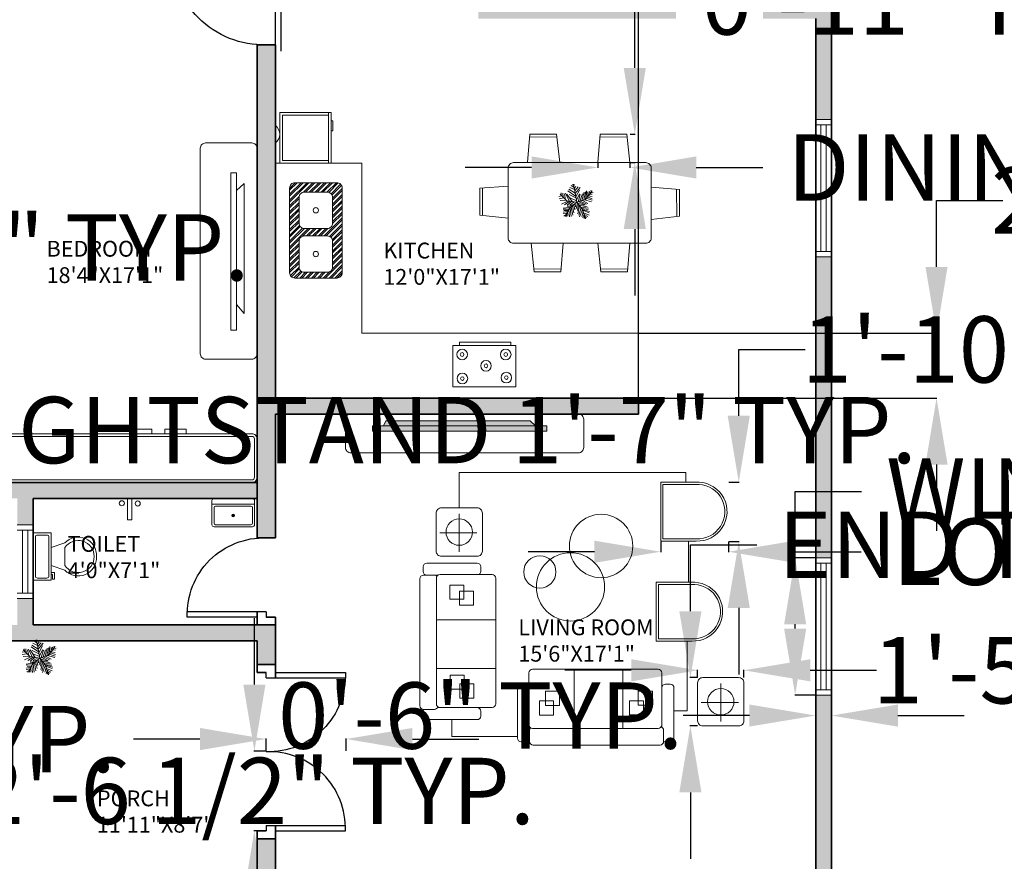
# Model space of a CAD drawing. Units: inches. Extents: x 35 to 5908, y 4 to 3165.
# Tile 3 of 6: x 5173 to 5546, y 2387 to 2706. Entities that reach past the tile are written whole.
import ezdxf

# ---------------------------------------------------------------- set-up
doc = ezdxf.new("R2010")
doc.units = ezdxf.units.IN
doc.header["$MEASUREMENT"] = 0
for name, color, linetype, lineweight in [('A-ANNO-DIMS', 2, 'Continuous', 18), ('A-DOOR', 4, 'Continuous', 25), ('A-FLOR-CASE', 8, 'Continuous', 18), ('A-FLOR-FIXT', 8, 'Continuous', 18), ('A-FURN', 8, 'Continuous', 18), ('A-FURN-PATT', 9, 'Continuous', 13), ('A-WALL', 7, 'Continuous', 35), ('A-WALL-PATT', 252, 'Continuous', 13), ('L-PLNT', 3, 'Continuous', 13)]:
    doc.layers.add(name, color=color, linetype=linetype, lineweight=lineweight)
for name, color, linetype, lineweight, true_color in [('A-AREA-IDEN', 30, 'Continuous', 18, 0xf8991e), ('A-EQPM', 41, 'Continuous', 18, 0xf4ee51), ('A-FIXT-PATT', 41, 'Continuous', 13, 0xf4ee51), ('A-GLAZ', 30, 'Continuous', 18, 0xf8991e)]:
    doc.layers.add(name, color=color, linetype=linetype, lineweight=lineweight, true_color=true_color)
doc.styles.get("Standard").update_dxf_attribs({"font": 'arial.ttf'})
doc.dimstyles.get("Standard").update_dxf_attribs({"dimtxt": 25.18, "dimasz": 25.18, "dimexe": 0.18, "dimexo": 0.0625, "dimgap": 0.09, "dimtad": 0, "dimtih": 1, "dimtoh": 1, "dimdec": 0, "dimzin": 0, "dimdsep": 46, "dimlunit": 3, "dimtxsty": 'Standard', "dimcen": 0.09, "dimadec": 0, "dimazin": 0, "dimtfac": 1, "dimtdec": 0, "dimtofl": 0, "dimtmove": 0, "dimatfit": 3, "dimfxl": 1, "dimtolj": 1, "dimtzin": 0, "dimarcsym": 0})

# ---------------------------------------------------------------- blocks, each defined once
blk = doc.blocks.new('*U2')
for p, q in [((-3.665, 19.273), (-27.574, 35.527)), ((-5.114, 28.097), (-24.676, 40.636)), ((-7.288, 39.707), (-21.778, 46.673)), ((-8.737, 47.138), (-17.069, 52.711)), ((-10.186, 53.64), (-13.084, 55.962)), ((0, 0), (-10.5, 57)), ((-9.099, 51.782), (-6.563, 55.962)), ((-7.65, 43.423), (-2.578, 49.46)), ((-5.839, 35.992), (4.667, 48.067)), ((-5.114, 27.632), (10.463, 46.673)), ((-2.941, 16.486), (8.652, 37.85)), ((16.259, 5.805), (23.142, 31.348)), ((22.055, 7.198), (27.489, 32.277)), ((27, 9), (48, 36)), ((27.127, 9.056), (31.112, 35.992)), ((35.096, 32.741), (37.27, 22.524)), ((38.719, 34.134), (41.979, 28.561)), ((44.153, 36.456), (45.239, 32.741)), ((-47.498, 19.737), (-55.83, 18.344)), ((-40.615, 13.7), (-55.105, 10.913)), ((-31.5, 4.5), (-52.5, 25.5)), ((-33.37, 6.269), (-52.207, 5.34)), ((-48.585, 21.131), (-49.309, 29.026)), ((-28.299, 3.483), (-47.86, -5.805)), ((-43.513, 28.561), (-42.427, 15.558)), ((-38.442, 26.239), (-34.819, 7.663)), ((-21.416, 3.018), (-38.079, -8.128)), ((-35.544, 28.097), (-24.314, 3.947)), ((0, 0), (-31.5, 4.5)), ((-14.533, 2.09), (-30.834, 25.31)), ((-15.982, 2.09), (-30.11, -9.521)), ((-24.314, 23.917), (-2.941, 13.7)), ((0, 0), (-22.5, -19.5)), ((-6.563, 1.161), (-21.416, -8.128)), ((-20.691, 13.7), (-1.129, 4.876)), ((-1.129, 6.734), (9.014, 26.704)), ((0, 0), (27, 9)), ((0, 0), (18, -22.5)), ((3.942, 1.625), (11.187, 24.381)), ((6.478, 1.625), (26.04, -8.592)), ((10.101, 3.483), (17.708, 26.239)), ((11.187, 3.483), (30.749, -5.805)), ((18.07, 5.805), (35.096, -3.483)), ((24.229, 7.663), (46.688, 1.625)), ((29.662, 12.307), (48.137, 6.269)), ((31.836, 30.883), (32.561, 16.486)), ((33.285, 16.486), (48.862, 10.913)), ((36.183, 19.737), (48.137, 17.88)), ((40.53, 25.775), (48.862, 24.846)), ((43.791, 29.954), (51.036, 30.883)), ((-17.431, -15.094), (-42.789, -18.809)), ((-28.299, -29.026), (-42.789, -31.348)), ((-24.314, -21.596), (-42.427, -22.06)), ((-26.849, -26.24), (-40.253, -25.775)), ((-22.5, -19.5), (-37.5, -45)), ((-15.257, -12.772), (-30.11, -12.772)), ((-29.023, -30.884), (-27.936, -43.887)), ((-25.038, -23.918), (-22.865, -45.281)), ((-20.691, -18.345), (-17.793, -44.352)), ((-6.563, -5.805), (-19.967, -9.985)), ((-17.069, -15.094), (-12.721, -40.172)), ((-13.446, -11.378), (-8.737, -32.741)), ((-9.461, -8.592), (-6.201, -23.453)), ((-4.752, -3.483), (-3.665, -14.629)), ((2.493, -3.019), (-1.491, -20.202)), ((1.769, -2.555), (24.229, -9.521)), ((5.029, -6.27), (2.131, -25.775)), ((9.014, -11.378), (3.58, -35.992)), ((14.085, -16.951), (6.478, -40.172)), ((7.565, -9.056), (32.198, -14.629)), ((18.07, -22.524), (8.289, -45.745)), ((12.274, -15.094), (36.907, -18.809)), ((20.244, -30.419), (15.897, -44.816)), ((16.259, -19.738), (36.183, -22.989)), ((18, -22.5), (27, -52.5)), ((18.433, -22.524), (40.53, -29.026)), ((19.157, -25.311), (38.719, -33.206)), ((-30.834, -34.135), (-42.427, -35.528)), ((-34.457, -39.708), (-40.978, -42.494)), ((-32.646, -36.921), (-31.921, -44.352)), ((22.78, -37.85), (19.519, -48.532)), ((21.331, -32.741), (39.081, -40.636)), ((22.78, -38.314), (34.372, -44.816)), ((24.591, -45.745), (23.142, -50.854)), ((24.591, -43.423), (30.749, -47.603)), ((26.764, -49.925), (28.213, -50.854))]:
    blk.add_line(p, q)
blk = doc.blocks.new('*U4')
for p, q in [((9.5, -6), (9.5, -2)), ((-10, -8.5), (-8, -8.5)), ((-10, -9.5), (-10, -8.5)), ((-8, -8.5), (-8, -8)), ((-7, -8), (-7, -9.5)), ((-4, -8), (-6, -14)), ((4, -8), (6, -14)), ((-7, -9.5), (-10, -9.5)), ((4, -14), (-4, -14))]:
    blk.add_line(p, q)
blk.add_lwpolyline([(10.5, -8), (10.5, 0), (-10.5, 0), (-10.5, -8)], close=True)
for points in [[(-9.5, -2), (-9.5, -6)], [(8.5, -1), (-8.5, -1)], [(-8.5, -7), (8.5, -7)]]:
    blk.add_lwpolyline(points)
for centre, radius, start, end in [((-8.625, -1.875), 0.8839, 81.8699, 188.1301), ((8.625, -1.875), 0.8839, 351.8699, 98.1301), ((-8.625, -6.125), 0.8839, 171.869898, 278.1301), ((8.625, -6.125), 0.8839, 261.8699, 8.1301), ((-0.4772, -19.9188), 8.0953, 133.01722, 273.38), ((0.0374, -19.8731), 7.127, 124.50543, 269.7), ((-0.0373, -19.8731), 7.127, 270.3, 55.4946), ((0.4773, -19.9188), 8.0953, 266.62, 46.9828)]:
    blk.add_arc(centre, radius, start, end)
blk = doc.blocks.new('Sink-single - 30 in top')
blk.add_line((-15, -3.999996), (15, -3.999996))
for points in [[(-13.5, 0), (13.5, 0)], [(-15, -18.499996), (-15, -1.5)], [(-13.5, -17.499996), (-13.5, -6.499996)], [(-12.5, -5.499996), (12.5, -5.499996)], [(13.5, -6.499996), (13.5, -17.499996)], [(15, -1.5), (15, -18.499996)], [(13.5, -19.999996), (-13.5, -19.999996)], [(12.5, -18.499996), (-12.5, -18.499996)]]:
    blk.add_lwpolyline(points)
for radius in [1, 0.5]:
    blk.add_circle((0, -11.999996), radius)
for centre, radius, start, end in [((-13.5, -1.5), 1.5, 90, 180), ((-12.5, -6.499996), 1, 90, 180), ((12.5, -6.499996), 1, 0, 90), ((13.5, -1.5), 1.5, 0, 90), ((-13.5, -18.499996), 1.5, 180, 270), ((-12.5, -17.499996), 1, 180, 270), ((12.5, -17.499996), 1, 270, 0), ((13.5, -18.499996), 1.5, 270, 0)]:
    blk.add_arc(centre, radius, start, end)
blk = doc.blocks.new('DOOR-30-3_5-JAMB')
for p, q in [((-3.5, 0), (-30, 0)), ((0, -2), (-30, -2)), ((0, -2), (0, 0))]:
    blk.add_line(p, q)
blk.add_arc((-1, -1), 29.02, 178.0251, 271.9749)
blk = doc.blocks.new('DOOR-36')
for p, q in [((0, 2), (-36, 2)), ((0, 2), (0, 0)), ((-3.5, 0), (-36, 0))]:
    blk.add_line(p, q)
blk.add_arc((-1, 1), 35.01, 88.3634, 181.6366)
blk = doc.blocks.new('WINDOW-48')
for p, q in [((0, 0), (0, 6)), ((2, 0), (2, 6)), ((2, 4), (50, 4)), ((50, 0), (50, 6)), ((52, 0), (52, 6)), ((2, 2), (50, 2))]:
    blk.add_line(p, q)
blk = doc.blocks.new('WINDOW-24')
for p, q in [((0, 0), (0, 6)), ((2, 0), (2, 6)), ((2, 4), (26, 4)), ((26, 0), (26, 6)), ((28, 0), (28, 6)), ((2, 2), (26, 2))]:
    blk.add_line(p, q)
blk = doc.blocks.new('CHAIR-DINING')
for p, q in [((0, 0), (0.86, 10.77)), ((0.78, 9.7), (11.11, 9.75)), ((0.86, 10.77), (11, 10.77)), ((11, 10.77), (12.18, 0))]:
    blk.add_line(p, q)
blk = doc.blocks.new('CHAIR-ROUND-BACK')
for p, q in [((14.57, 22.32), (0, 22.32)), ((0, 22.32), (0, 0.01)), ((0.83, 21.49), (0.83, 0.84)), ((14.57, 21.49), (0.83, 21.49)), ((13.44, 0.01), (0, 0.01)), ((13.44, 0.84), (0.83, 0.84))]:
    blk.add_line(p, q)
for radius in [11.17, 10.34]:
    blk.add_arc((14.01, 11.17), radius, 267.0936, 87.0936)
blk = doc.blocks.new('TABLE-LAMP-END')
for p, q in [((0, 6.97), (0, -7.48)), ((-7.39, -0.25), (6.7, -0.25))]:
    blk.add_line(p, q)
blk.add_lwpolyline([(-8.78, 7.18, -0.414214), (-6.78, 9.18), (6.78, 9.18, -0.414214), (8.78, 7.18), (8.78, -7.18, -0.414214), (6.78, -9.18), (-6.78, -9.18, -0.414214), (-8.78, -7.18)], format="xyb", close=True)
blk.add_circle((0, 0), 5.01)
blk = doc.blocks.new('*D20')
at = {"layer": 'A-ANNO-DIMS', "color": 0, "lineweight": -2, "transparency": 16777216}
for p, q in [((5366.93, 2650.28), (5341.75, 2650.28)), ((5392.11, 2652.05), (5392.11, 2650.1)), ((5404.3, 2652.05), (5404.3, 2650.1)), ((5429.48, 2650.28), (5454.66, 2650.28))]:
    blk.add_line(p, q, dxfattribs=at)
for points in [[(5366.93, 2654.48), (5366.93, 2646.08), (5392.11, 2650.28)], [(5429.48, 2654.48), (5429.48, 2646.08), (5404.3, 2650.28)]]:
    blk.add_solid(points, dxfattribs=at)
at = {"layer": 'Defpoints', "color": 0, "lineweight": -2, "transparency": 16777216}
for p in [(5392.11, 2652.11), (5404.3, 2652.11), (5404.3, 2650.28)]:
    blk.add_point(p, dxfattribs=at)
at = {"layer": 'A-ANNO-DIMS', "color": 0, "transparency": 16777216, "insert": (5656.92, 2650.28), "char_height": 25.18, "attachment_point": 5}
blk.add_mtext('\\A1;DINING CHAIR 1\'-0" TYP.', dxfattribs=at)
blk = doc.blocks.new('*D21')
at = {"layer": 'A-ANNO-DIMS', "color": 0, "lineweight": -2, "transparency": 16777216}
for p, q in [((5406.13, 2688.06), (5406.13, 2713.24)), ((5406.13, 2713.24), (5431.31, 2713.24)), ((5404.36, 2662.88), (5406.31, 2662.88)), ((5404.36, 2652.11), (5406.31, 2652.11)), ((5406.13, 2626.93), (5406.13, 2601.75))]:
    blk.add_line(p, q, dxfattribs=at)
for points in [[(5401.93, 2688.06), (5410.32, 2688.06), (5406.13, 2662.88)], [(5401.93, 2626.93), (5410.32, 2626.93), (5406.13, 2652.11)]]:
    blk.add_solid(points, dxfattribs=at)
at = {"layer": 'Defpoints', "color": 0, "lineweight": -2, "transparency": 16777216}
for p in [(5404.3, 2662.88), (5406.13, 2662.88), (5404.3, 2652.11)]:
    blk.add_point(p, dxfattribs=at)
at = {"layer": 'A-ANNO-DIMS', "color": 0, "transparency": 16777216, "insert": (5517.92, 2713.24), "char_height": 25.18, "attachment_point": 5}
blk.add_mtext('\\A1;0\'-11" TYP.', dxfattribs=at)
blk = doc.blocks.new('*D22')
at = {"layer": 'A-ANNO-DIMS', "color": 0, "lineweight": -2, "transparency": 16777216}
for p, q in [((5466.99, 2502.2), (5466.99, 2527.38)), ((5466.99, 2527.38), (5492.17, 2527.38)), ((5474.73, 2502.2), (5466.81, 2502.2)), ((5466.99, 2475.38), (5466.99, 2477.02)), ((5474.73, 2450.2), (5466.81, 2450.2))]:
    blk.add_line(p, q, dxfattribs=at)
for points in [[(5462.8, 2477.02), (5471.19, 2477.02), (5466.99, 2502.2)], [(5462.8, 2475.38), (5471.19, 2475.38), (5466.99, 2450.2)]]:
    blk.add_solid(points, dxfattribs=at)
at = {"layer": 'Defpoints', "color": 0, "lineweight": -2, "transparency": 16777216}
for p in [(5466.99, 2502.2), (5474.79, 2502.2), (5474.79, 2450.2)]:
    blk.add_point(p, dxfattribs=at)
at = {"layer": 'A-ANNO-DIMS', "color": 0, "transparency": 16777216, "insert": (5682.85, 2527.38), "char_height": 25.18, "attachment_point": 5}
blk.add_mtext('\\A1;WINDOW W1 4\'-4" TYP.', dxfattribs=at)
blk = doc.blocks.new('*D23')
at = {"layer": 'A-ANNO-DIMS', "color": 0, "lineweight": -2, "transparency": 16777216}
for p, q in [((5474.79, 2450.14), (5474.79, 2442.22)), ((5480.79, 2450.14), (5480.79, 2442.22)), ((5449.61, 2442.4), (5424.43, 2442.4)), ((5505.97, 2442.4), (5531.15, 2442.4))]:
    blk.add_line(p, q, dxfattribs=at)
for points in [[(5449.61, 2446.6), (5449.61, 2438.21), (5474.79, 2442.4)], [(5505.97, 2446.6), (5505.97, 2438.21), (5480.79, 2442.4)]]:
    blk.add_solid(points, dxfattribs=at)
at = {"layer": 'Defpoints', "color": 0, "lineweight": -2, "transparency": 16777216}
for p in [(5474.79, 2450.2), (5480.79, 2450.2), (5474.79, 2442.4)]:
    blk.add_point(p, dxfattribs=at)
at = {"layer": 'A-ANNO-DIMS', "color": 0, "transparency": 16777216, "insert": (5347.6, 2442.4), "char_height": 25.18, "attachment_point": 5}
blk.add_mtext('\\A1;0\'-6" TYP.', dxfattribs=at)
blk = doc.blocks.new('*D26')
at = {"layer": 'A-ANNO-DIMS', "color": 0, "lineweight": -2, "transparency": 16777216}
for p, q in [((5241.11, 2433.5), (5215.93, 2433.5)), ((5266.29, 2429.02), (5266.29, 2433.68)), ((5296.57, 2429.02), (5296.57, 2433.68)), ((5321.75, 2433.5), (5346.93, 2433.5))]:
    blk.add_line(p, q, dxfattribs=at)
for points in [[(5241.11, 2437.7), (5241.11, 2429.3), (5266.29, 2433.5)], [(5321.75, 2437.7), (5321.75, 2429.3), (5296.57, 2433.5)]]:
    blk.add_solid(points, dxfattribs=at)
at = {"layer": 'Defpoints', "color": 0, "lineweight": -2, "transparency": 16777216}
for p in [(5266.29, 2433.5), (5266.29, 2428.96), (5296.57, 2428.96)]:
    blk.add_point(p, dxfattribs=at)
at = {"layer": 'A-ANNO-DIMS', "color": 0, "transparency": 16777216, "insert": (5025.37, 2433.5), "char_height": 25.18, "attachment_point": 5}
blk.add_mtext('\\A1;DOOR D1 2\'-6 1/2" TYP.', dxfattribs=at)
blk = doc.blocks.new('*D27')
at = {"layer": 'A-ANNO-DIMS', "color": 0, "lineweight": -2, "transparency": 16777216}
for p, q in [((5261.75, 2454.14), (5261.75, 2479.32)), ((5266.23, 2428.96), (5261.57, 2428.96)), ((5266.23, 2398.68), (5261.57, 2398.68)), ((5261.75, 2373.5), (5261.75, 2348.32))]:
    blk.add_line(p, q, dxfattribs=at)
for points in [[(5257.56, 2454.14), (5265.95, 2454.14), (5261.75, 2428.96)], [(5257.56, 2373.5), (5265.95, 2373.5), (5261.75, 2398.68)]]:
    blk.add_solid(points, dxfattribs=at)
at = {"layer": 'Defpoints', "color": 0, "lineweight": -2, "transparency": 16777216}
for p in [(5266.29, 2428.96), (5261.75, 2398.68), (5266.29, 2398.68)]:
    blk.add_point(p, dxfattribs=at)
at = {"layer": 'A-ANNO-DIMS', "color": 0, "transparency": 16777216, "insert": (5261.75, 2413.82), "char_height": 25.18, "attachment_point": 5}
blk.add_mtext('\\A1;2\'-6 1/2" TYP.', dxfattribs=at)
blk = doc.blocks.new('*D32')
at = {"layer": 'A-ANNO-DIMS', "color": 0, "lineweight": -2, "transparency": 16777216}
for p, q in [((5230.02, 2744.72), (5230.02, 2739.16)), ((5266.29, 2744.72), (5266.29, 2739.16)), ((5204.84, 2739.34), (5179.66, 2739.34)), ((5291.47, 2739.34), (5316.65, 2739.34))]:
    blk.add_line(p, q, dxfattribs=at)
for points in [[(5204.84, 2743.53), (5204.84, 2735.14), (5230.02, 2739.34)], [(5291.47, 2743.53), (5291.47, 2735.14), (5266.29, 2739.34)]]:
    blk.add_solid(points, dxfattribs=at)
at = {"layer": 'Defpoints', "color": 0, "lineweight": -2, "transparency": 16777216}
for p in [(5230.02, 2744.78), (5266.29, 2744.78), (5266.29, 2739.34)]:
    blk.add_point(p, dxfattribs=at)
at = {"layer": 'A-ANNO-DIMS', "color": 0, "transparency": 16777216, "insert": (5507.22, 2739.34), "char_height": 25.18, "attachment_point": 5}
blk.add_mtext('\\A1;DOOR D3 3\'-0 1/2" TYP.', dxfattribs=at)
blk = doc.blocks.new('*D33')
at = {"layer": 'A-ANNO-DIMS', "color": 0, "lineweight": -2, "transparency": 16777216}
for p, q in [((5271.74, 2806.23), (5271.74, 2831.41)), ((5266.36, 2781.05), (5271.92, 2781.05)), ((5266.36, 2744.78), (5271.92, 2744.78)), ((5271.74, 2719.6), (5271.74, 2694.42))]:
    blk.add_line(p, q, dxfattribs=at)
for points in [[(5267.54, 2806.23), (5275.93, 2806.23), (5271.74, 2781.05)], [(5267.54, 2719.6), (5275.93, 2719.6), (5271.74, 2744.78)]]:
    blk.add_solid(points, dxfattribs=at)
at = {"layer": 'Defpoints', "color": 0, "lineweight": -2, "transparency": 16777216}
for p in [(5266.29, 2781.05), (5271.74, 2781.05), (5266.29, 2744.78)]:
    blk.add_point(p, dxfattribs=at)
at = {"layer": 'A-ANNO-DIMS', "color": 0, "transparency": 16777216, "insert": (5271.74, 2762.92), "char_height": 25.18, "attachment_point": 5}
blk.add_mtext('\\A1;3\'-0 1/2" TYP.', dxfattribs=at)
blk = doc.blocks.new('*D38')
at = {"layer": 'A-ANNO-DIMS', "color": 0, "lineweight": -2, "transparency": 16777216}
for p, q in [((5060.55, 2553.45), (5060.55, 2550.51)), ((5079.39, 2553.45), (5079.39, 2550.51)), ((5035.37, 2550.69), (5010.19, 2550.69)), ((5104.57, 2550.69), (5129.75, 2550.69))]:
    blk.add_line(p, q, dxfattribs=at)
for points in [[(5035.37, 2554.88), (5035.37, 2546.49), (5060.55, 2550.69)], [(5104.57, 2554.88), (5104.57, 2546.49), (5079.39, 2550.69)]]:
    blk.add_solid(points, dxfattribs=at)
at = {"layer": 'Defpoints', "color": 0, "lineweight": -2, "transparency": 16777216}
for p in [(5060.55, 2553.51), (5079.39, 2553.51), (5079.39, 2550.69)]:
    blk.add_point(p, dxfattribs=at)
at = {"layer": 'A-ANNO-DIMS', "color": 0, "transparency": 16777216, "insert": (5325.18, 2550.69), "char_height": 25.18, "attachment_point": 5}
blk.add_mtext('\\A1;NIGHTSTAND 1\'-7" TYP.', dxfattribs=at)
blk = doc.blocks.new('*D39')
at = {"layer": 'A-ANNO-DIMS', "color": 0, "lineweight": -2, "transparency": 16777216}
for p, q in [((5082.21, 2594.78), (5082.21, 2619.96)), ((5082.21, 2619.96), (5107.39, 2619.96)), ((5079.45, 2569.6), (5082.39, 2569.6)), ((5079.45, 2553.51), (5082.39, 2553.51)), ((5082.21, 2528.33), (5082.21, 2503.15))]:
    blk.add_line(p, q, dxfattribs=at)
for points in [[(5078.01, 2594.78), (5086.41, 2594.78), (5082.21, 2569.6)], [(5078.01, 2528.33), (5086.41, 2528.33), (5082.21, 2553.51)]]:
    blk.add_solid(points, dxfattribs=at)
at = {"layer": 'Defpoints', "color": 0, "lineweight": -2, "transparency": 16777216}
for p in [(5079.39, 2569.6), (5082.21, 2569.6), (5079.39, 2553.51)]:
    blk.add_point(p, dxfattribs=at)
at = {"layer": 'A-ANNO-DIMS', "color": 0, "transparency": 16777216, "insert": (5183.04, 2619.96), "char_height": 25.18, "attachment_point": 5}
blk.add_mtext('\\A1;1\'-4" TYP.', dxfattribs=at)
blk = doc.blocks.new('*D42')
at = {"layer": 'A-ANNO-DIMS', "color": 0, "lineweight": -2, "transparency": 16777216}
for p, q in [((5415.96, 2508.34), (5415.96, 2504.36)), ((5441.72, 2508.34), (5441.72, 2504.36)), ((5390.78, 2504.54), (5365.6, 2504.54)), ((5466.9, 2504.54), (5492.08, 2504.54))]:
    blk.add_line(p, q, dxfattribs=at)
for points in [[(5390.78, 2508.73), (5390.78, 2500.34), (5415.96, 2504.54)], [(5466.9, 2508.73), (5466.9, 2500.34), (5441.72, 2504.54)]]:
    blk.add_solid(points, dxfattribs=at)
at = {"layer": 'Defpoints', "color": 0, "lineweight": -2, "transparency": 16777216}
for p in [(5415.96, 2508.4), (5441.72, 2508.4), (5441.72, 2504.54)]:
    blk.add_point(p, dxfattribs=at)
at = {"layer": 'A-ANNO-DIMS', "color": 0, "transparency": 16777216, "insert": (5707.13, 2504.54), "char_height": 25.18, "attachment_point": 5}
blk.add_mtext('\\A1;LOUNGE CHAIR 2\'-2" TYP.', dxfattribs=at)
blk = doc.blocks.new('*D43')
at = {"layer": 'A-ANNO-DIMS', "color": 0, "lineweight": -2, "transparency": 16777216}
for p, q in [((5445.59, 2556.09), (5445.59, 2581.27)), ((5445.59, 2581.27), (5470.77, 2581.27)), ((5441.78, 2530.91), (5445.77, 2530.91)), ((5441.78, 2508.4), (5445.77, 2508.4)), ((5445.59, 2483.22), (5445.59, 2458.04))]:
    blk.add_line(p, q, dxfattribs=at)
for points in [[(5441.39, 2556.09), (5449.78, 2556.09), (5445.59, 2530.91)], [(5441.39, 2483.22), (5449.78, 2483.22), (5445.59, 2508.4)]]:
    blk.add_solid(points, dxfattribs=at)
at = {"layer": 'Defpoints', "color": 0, "lineweight": -2, "transparency": 16777216}
for p in [(5441.72, 2530.91), (5445.59, 2530.91), (5441.72, 2508.4)]:
    blk.add_point(p, dxfattribs=at)
at = {"layer": 'A-ANNO-DIMS', "color": 0, "transparency": 16777216, "insert": (5585.53, 2581.27), "char_height": 25.18, "attachment_point": 5}
blk.add_mtext('\\A1;1\'-10 1/2" TYP.', dxfattribs=at)
blk = doc.blocks.new('*D44')
at = {"layer": 'A-ANNO-DIMS', "color": 0, "lineweight": -2, "transparency": 16777216}
for p, q in [((5427.23, 2481.99), (5427.23, 2507.17)), ((5427.23, 2507.17), (5452.41, 2507.17)), ((5429.92, 2456.81), (5427.05, 2456.81)), ((5429.92, 2438.45), (5427.05, 2438.45)), ((5427.23, 2413.27), (5427.23, 2388.09))]:
    blk.add_line(p, q, dxfattribs=at)
for points in [[(5423.03, 2481.99), (5431.43, 2481.99), (5427.23, 2456.81)], [(5423.03, 2413.27), (5431.43, 2413.27), (5427.23, 2438.45)]]:
    blk.add_solid(points, dxfattribs=at)
at = {"layer": 'Defpoints', "color": 0, "lineweight": -2, "transparency": 16777216}
for p in [(5427.23, 2456.81), (5429.99, 2456.81), (5429.99, 2438.45)]:
    blk.add_point(p, dxfattribs=at)
at = {"layer": 'A-ANNO-DIMS', "color": 0, "transparency": 16777216, "insert": (5660.55, 2507.17), "char_height": 25.18, "attachment_point": 5}
blk.add_mtext('\\A1;END TABLE 1\'-6 1/2" TYP.', dxfattribs=at)
blk = doc.blocks.new('*D45')
at = {"layer": 'A-ANNO-DIMS', "color": 0, "lineweight": -2, "transparency": 16777216}
for p, q in [((5404.81, 2459.57), (5379.63, 2459.57)), ((5429.99, 2456.88), (5429.99, 2459.75)), ((5447.54, 2456.88), (5447.54, 2459.75)), ((5472.72, 2459.57), (5497.9, 2459.57))]:
    blk.add_line(p, q, dxfattribs=at)
for points in [[(5404.81, 2463.77), (5404.81, 2455.37), (5429.99, 2459.57)], [(5472.72, 2463.77), (5472.72, 2455.37), (5447.54, 2459.57)]]:
    blk.add_solid(points, dxfattribs=at)
at = {"layer": 'Defpoints', "color": 0, "lineweight": -2, "transparency": 16777216}
for p in [(5447.54, 2459.57), (5429.99, 2456.81), (5447.54, 2456.81)]:
    blk.add_point(p, dxfattribs=at)
at = {"layer": 'A-ANNO-DIMS', "color": 0, "transparency": 16777216, "insert": (5602.88, 2459.57), "char_height": 25.18, "attachment_point": 5}
blk.add_mtext('\\A1;1\'-5 1/2" TYP.', dxfattribs=at)
blk = doc.blocks.new('*D50')
at = {"layer": 'A-ANNO-DIMS', "color": 0, "lineweight": -2, "transparency": 16777216}
for p, q in [((5269.79, 2562.84), (5269.79, 3127.3)), ((5294.97, 3127.12), (5382.35, 3127.12)), ((5407.53, 2562.84), (5407.53, 3127.3)), ((5407.53, 3127.12), (5432.71, 3127.12))]:
    blk.add_line(p, q, dxfattribs=at)
for points in [[(5294.97, 3131.32), (5294.97, 3122.92), (5269.79, 3127.12)], [(5382.35, 3131.32), (5382.35, 3122.92), (5407.53, 3127.12)]]:
    blk.add_solid(points, dxfattribs=at)
at = {"layer": 'Defpoints', "color": 0, "lineweight": -2, "transparency": 16777216}
for p in [(5407.53, 3127.12), (5269.79, 2562.78), (5407.53, 2562.78)]:
    blk.add_point(p, dxfattribs=at)
at = {"layer": 'A-ANNO-DIMS', "color": 0, "transparency": 16777216, "insert": (5504.2, 3127.12), "char_height": 25.18, "attachment_point": 5}
blk.add_mtext('\\A1;11\'-5 1/2"', dxfattribs=at)
blk = doc.blocks.new('*D51')
at = {"layer": 'A-ANNO-DIMS', "color": 0, "lineweight": -2, "transparency": 16777216}
for p, q in [((5520.64, 2612.59), (5520.64, 2637.77)), ((5520.64, 2637.77), (5545.82, 2637.77)), ((5407.59, 2587.41), (5520.82, 2587.41)), ((5407.59, 2562.78), (5520.82, 2562.78)), ((5520.64, 2537.6), (5520.64, 2512.42))]:
    blk.add_line(p, q, dxfattribs=at)
for points in [[(5516.45, 2612.59), (5524.84, 2612.59), (5520.64, 2587.41)], [(5516.45, 2537.6), (5524.84, 2537.6), (5520.64, 2562.78)]]:
    blk.add_solid(points, dxfattribs=at)
at = {"layer": 'Defpoints', "color": 0, "lineweight": -2, "transparency": 16777216}
for p in [(5407.53, 2587.41), (5520.64, 2587.41), (5407.53, 2562.78)]:
    blk.add_point(p, dxfattribs=at)
at = {"layer": 'A-ANNO-DIMS', "color": 0, "transparency": 16777216, "insert": (5608.93, 2637.77), "char_height": 25.18, "attachment_point": 5}
blk.add_mtext('\\A1;2\'-0 1/2"', dxfattribs=at)

msp = doc.modelspace()

# ---------------------------------------------------------------- hatches: boundary and pattern name
at = {"layer": 'A-FIXT-PATT'}
h = msp.add_hatch(dxfattribs=at)
h.set_pattern_fill('ANSI32', color=256, scale=4.2)
h.paths.add_polyline_path([(5293.08, 2644.5), (5277.13, 2644.5, 0.414214), (5275.13, 2642.5), (5275.13, 2610.35, 0.414214), (5277.13, 2608.35), (5293.08, 2608.35, 0.414214), (5295.08, 2610.35), (5295.08, 2642.5, 0.414214)])
h.paths.add_polyline_path([(5280.69, 2640.92), (5289.46, 2640.92, -0.414214), (5291.46, 2638.92), (5291.46, 2629.16, -0.414214), (5289.46, 2627.16), (5280.69, 2627.16, -0.414214), (5278.69, 2629.16), (5278.69, 2638.92, -0.414214)], flags=16)
h.paths.add_polyline_path([(5286.09, 2634.04, -1), (5284.06, 2634.04, -1)], flags=0)
h.paths.add_polyline_path([(5280.69, 2624.32), (5289.46, 2624.32, -0.414214), (5291.46, 2622.32), (5291.46, 2612.55, -0.414214), (5289.46, 2610.55), (5280.69, 2610.55, -0.414214), (5278.69, 2612.55), (5278.69, 2622.32, -0.414214)], flags=16)
h.paths.add_polyline_path([(5286.09, 2617.44, -1), (5284.06, 2617.44, -1)], flags=0)
at = {"layer": 'A-FURN-PATT'}
h = msp.add_hatch(color=256, dxfattribs=at)
h.dxf.hatch_style = 1
h.paths.add_polyline_path([(5372.79, 2552.26), (5306.59, 2552.26), (5306.59, 2550.25), (5372.79, 2550.25)])
h.paths.add_polyline_path([(5366.47, 2554.2), (5311.65, 2554.2), (5310.73, 2552.26), (5368.44, 2552.26)])
at = {"layer": 'A-WALL-PATT'}
h = msp.add_hatch(color=256, dxfattribs=at)
h.dxf.hatch_style = 1
h.paths.add_polyline_path([(5198.29, 3041.78), (5119.29, 3041.78), (5119.29, 3035.78), (5155.79, 3035.78), (5155.79, 2967.78), (5087.79, 2967.78), (5087.79, 2966.78, -0.017236), (5087.79, 2964.78), (5087.79, 2961.78), (5262.79, 2961.78), (5262.79, 2967.78), (5236.55, 2967.78), (5236.55, 2967.75), (5218.53, 2967.75), (5161.79, 2967.78), (5161.79, 3035.78), (5198.29, 3035.78)])
h.paths.add_polyline_path([(5091.29, 3041.78), (5048.79, 3041.78), (5048.79, 2877.78), (5054.79, 2877.78), (5054.79, 2899), (5054.79, 2961.78), (5054.79, 2967.78), (5054.79, 3035.78), (5091.29, 3035.78)])
h.paths.add_polyline_path([(5346.29, 3041.78), (5226.29, 3041.78), (5226.29, 3035.78), (5262.79, 3035.78), (5269.79, 3035.78), (5346.29, 3035.78)])
h.paths.add_polyline_path([(5480.79, 3041.78), (5398.29, 3041.78), (5398.29, 3035.78), (5407.91, 3035.78), (5474.79, 3035.78), (5474.79, 2807.78), (5269.79, 2807.78), (5269.79, 3002.78), (5266.29, 3002.78, -0.017236), (5264.29, 3002.78), (5262.79, 3002.78), (5262.79, 2967.78), (5262.79, 2961.78), (5262.79, 2780.78), (5264.29, 2780.78, -0.014283), (5266.29, 2780.78), (5269.79, 2780.78), (5269.79, 2801.78), (5412.79, 2801.78), (5412.79, 2712.78), (5346.79, 2712.78), (5346.79, 2706.78), (5421.79, 2706.78), (5421.79, 2709.78, -0.017236), (5421.79, 2711.78), (5421.79, 2712.78), (5418.79, 2712.78), (5418.79, 2801.78), (5474.79, 2801.78), (5474.79, 2712.78), (5454.79, 2712.78), (5454.79, 2706.78), (5474.79, 2706.78), (5474.79, 2668.42), (5480.79, 2668.42)])
h.paths.add_polyline_path([(5054.79, 2825.78), (5048.79, 2825.78), (5048.79, 2632.28), (5054.79, 2632.28), (5054.79, 2642.69), (5054.79, 2735.78), (5262.79, 2735.78), (5262.79, 2741.78), (5054.79, 2741.78)])
h.paths.add_polyline_path([(5480.79, 2616.42), (5474.79, 2616.42), (5474.79, 2502.2), (5480.79, 2502.2)])
h.paths.add_polyline_path([(5407.53, 2562.78), (5269.79, 2562.78), (5269.79, 2696.78), (5266.29, 2696.78, -0.014283), (5264.29, 2696.78), (5262.79, 2696.78), (5262.79, 2509.78), (5264.29, 2509.78, -0.017236), (5266.29, 2509.78), (5269.79, 2509.78), (5269.79, 2556.78), (5407.53, 2556.78)])
h.paths.add_polyline_path([(5262.79, 2530.78), (5087.79, 2530.78), (5087.79, 2527.78, -0.017236), (5087.79, 2525.78), (5087.79, 2524.78), (5143.79, 2524.78), (5143.79, 2514.78), (5149.79, 2514.78), (5149.79, 2524.78), (5171.79, 2524.78), (5171.79, 2514.78), (5177.79, 2514.78), (5177.79, 2524.78), (5262.79, 2524.78)], flags=17)
h.paths.add_polyline_path([(5262.79, 2395.71), (5262.79, 2321.78), (5480.79, 2321.78), (5480.79, 2450.2), (5474.79, 2450.2), (5474.79, 2381.78), (5425.29, 2381.78), (5425.29, 2375.78), (5474.79, 2375.78), (5474.79, 2327.78), (5269.79, 2327.78), (5269.79, 2375.78), (5312.61, 2375.78), (5312.61, 2381.78), (5269.79, 2381.78), (5269.79, 2395.71)])
h.paths.add_polyline_path([(5171.13, 2321.78), (5171.13, 2327.78), (5054.79, 2327.78), (5054.79, 2470.78), (5157.79, 2470.78), (5262.79, 2470.78), (5262.79, 2461.71), (5269.79, 2461.71), (5269.79, 2476.78), (5262.79, 2476.78), (5177.79, 2476.78), (5177.79, 2486.78), (5171.79, 2486.78), (5171.79, 2476.78), (5149.79, 2476.78), (5149.79, 2486.78), (5143.79, 2486.78), (5143.79, 2476.78), (5054.79, 2476.78), (5054.79, 2580.28), (5048.79, 2580.28), (5048.79, 2321.78)])

# ---------------------------------------------------------------- linework, layer by layer
at = {"layer": 'A-DOOR'}
for p, q in [((5269.79, 2428.71), (5266.29, 2428.71)), ((5269.79, 2428.8), (5269.79, 2428.59))]:
    msp.add_line(p, q, dxfattribs=at)
at = {"layer": 'A-EQPM'}
for p, q in [((5289.91, 2670.12), (5289.91, 2671.12)), ((5289.91, 2652.94), (5289.91, 2651.94))]:
    msp.add_line(p, q, dxfattribs=at)
for points in [[(5269.79, 2670.8), (5269.79, 2670.8), (5269.79, 2661.59), (5269.79, 2661.59)], [(5271.37, 2671.12), (5290.91, 2671.12), (5290.91, 2651.94), (5271.37, 2651.94)], [(5272.37, 2670.12), (5289.91, 2670.12), (5289.91, 2652.94), (5272.37, 2652.94)], [(5290.91, 2668.01), (5291.47, 2668.01), (5291.47, 2664.23), (5290.91, 2664.23)], [(5337.01, 2582.77), (5337.01, 2582.77), (5361, 2582.77), (5361, 2582.77), (5361, 2567.04), (5361, 2567.04), (5337.01, 2567.04), (5337.01, 2567.04)], [(5339.66, 2582.77), (5339.66, 2582.77), (5359.03, 2582.77), (5359.03, 2582.77), (5359.03, 2584.03), (5359.03, 2584.03), (5339.66, 2584.03), (5339.66, 2584.03)]]:
    msp.add_lwpolyline(points, close=True, dxfattribs=at)
for centre, radius in [((5340.59, 2579.35), 2.02), ((5340.59, 2579.35), 0.697), ((5357.15, 2579.35), 2.02), ((5357.15, 2579.35), 0.697), ((5349.66, 2575.05), 2.02), ((5349.66, 2575.05), 0.697), ((5340.69, 2570.24), 2.02), ((5340.69, 2570.24), 0.697), ((5357.38, 2570.59), 2.02), ((5357.38, 2570.59), 0.697)]:
    msp.add_circle(centre, radius, dxfattribs=at)
msp.add_arc((5267.1, 2662.89), 4.27, 309.1488, 50.8512, dxfattribs=at)
at = {"layer": 'A-FLOR-CASE'}
for p, q in [((5269.79, 2651.94), (5269.79, 2651.94)), ((5269.79, 2651.94), (5302.52, 2651.94)), ((5302.52, 2651.94), (5302.52, 2587.41)), ((5302.52, 2587.41), (5407.53, 2587.41)), ((5407.53, 2587.41), (5407.53, 2562.78))]:
    msp.add_line(p, q, dxfattribs=at)
for points in [[(5262.79, 2532.78, -0.414214), (5260.79, 2530.78), (5120.49, 2530.78, -0.414214), (5118.49, 2532.78), (5118.49, 2547.31, -0.414214), (5120.49, 2549.31), (5260.79, 2549.31, -0.414214), (5262.79, 2547.31)], [(5261.79, 2532.78, -0.414214), (5260.79, 2531.78), (5120.49, 2531.78, -0.414214), (5119.49, 2532.78), (5119.49, 2547.31, -0.414214), (5120.49, 2548.31), (5260.79, 2548.31, -0.414214), (5261.79, 2547.31)]]:
    msp.add_lwpolyline(points, format="xyb", close=True, dxfattribs=at)
for points in [[(5214.73, 2549.31), (5214.73, 2549.31), (5222.81, 2549.31), (5222.81, 2549.31), (5222.81, 2551.08), (5222.81, 2551.08), (5214.73, 2551.08), (5214.73, 2551.08)], [(5227.77, 2549.31), (5227.77, 2549.31), (5235.85, 2549.31), (5235.85, 2549.31), (5235.85, 2551.08), (5235.85, 2551.08), (5227.77, 2551.08), (5227.77, 2551.08)]]:
    msp.add_lwpolyline(points, close=True, dxfattribs=at)
at = {"layer": 'A-FLOR-FIXT'}
for points in [[(5275.13, 2642.5, -0.414214), (5277.13, 2644.5), (5293.08, 2644.5, -0.414214), (5295.08, 2642.5), (5295.08, 2610.35, -0.414214), (5293.08, 2608.35), (5277.13, 2608.35, -0.414214), (5275.13, 2610.35)], [(5278.69, 2638.92, -0.414214), (5280.69, 2640.92), (5289.46, 2640.92, -0.414214), (5291.46, 2638.92), (5291.46, 2629.16, -0.414214), (5289.46, 2627.16), (5280.69, 2627.16, -0.414214), (5278.69, 2629.16)], [(5278.69, 2622.32, -0.414214), (5280.69, 2624.32), (5289.46, 2624.32, -0.414214), (5291.46, 2622.32), (5291.46, 2612.55, -0.414214), (5289.46, 2610.55), (5280.69, 2610.55, -0.414214), (5278.69, 2612.55)]]:
    msp.add_lwpolyline(points, format="xyb", close=True, dxfattribs=at)
msp.add_lwpolyline([(5215.22, 2524.78), (5215.22, 2524.78), (5213.66, 2524.78), (5213.66, 2524.78), (5213.66, 2516.58), (5213.66, 2516.58), (5215.22, 2516.58), (5215.22, 2516.58)], close=True, dxfattribs=at)
for centre, radius in [((5285.08, 2634.04), 1.02), ((5285.08, 2617.44), 1.02), ((5211.45, 2522.92), 0.954), ((5217.48, 2522.84), 0.954)]:
    msp.add_circle(centre, radius, dxfattribs=at)
at = {"layer": 'A-FURN'}
for p, q in [((5255.02, 2641.5), (5257.9, 2644.24)), ((5257.9, 2644.24), (5257.9, 2594.95)), ((5257.9, 2594.95), (5255.02, 2598.33)), ((5310.73, 2552.26), (5311.65, 2554.2)), ((5311.65, 2554.2), (5366.47, 2554.2)), ((5366.47, 2554.2), (5368.44, 2552.26)), ((5339.51, 2528.06), (5339.51, 2534.64)), ((5339.51, 2534.64), (5425.45, 2534.64)), ((5425.45, 2534.64), (5425.45, 2530.91)), ((5339.51, 2521.18), (5339.51, 2528.06)), ((5426.45, 2508.6), (5426.45, 2492.97)), ((5330.83, 2478.71), (5353.35, 2478.71)), ((5425.98, 2470.66), (5425.98, 2444.21)), ((5330.83, 2460.23), (5353.35, 2460.23)), ((5383.13, 2437.48), (5383.13, 2460.01)), ((5401.61, 2437.48), (5401.61, 2460.01)), ((5425.98, 2444.21), (5421, 2444.21)), ((5336.74, 2440.85), (5336.74, 2434.49)), ((5336.74, 2434.49), (5361.61, 2434.49))]:
    msp.add_line(p, q, dxfattribs=at)
for points in [[(5262.79, 2657.58, 0.414214), (5260.79, 2659.58), (5243.24, 2659.58, 0.414214), (5241.24, 2657.58), (5241.24, 2579.6, 0.414214), (5243.24, 2577.6), (5260.79, 2577.6, 0.414214), (5262.79, 2579.6)], [(5358.08, 2650.11, -0.414214), (5360.08, 2652.11), (5410.32, 2652.11, -0.414214), (5412.32, 2650.11), (5412.32, 2623.52, -0.414214), (5410.32, 2621.52), (5360.08, 2621.52, -0.414214), (5358.08, 2623.52)], [(5296.32, 2554.78, -0.414214), (5298.32, 2556.78), (5384.75, 2556.78, -0.414214), (5386.75, 2554.78), (5386.75, 2544.06, -0.414214), (5384.75, 2542.06), (5298.32, 2542.06, -0.414214), (5296.32, 2544.06)], [(5353.35, 2494.5, 0.414214), (5351.97, 2495.88), (5332.21, 2495.88, 0.414214), (5330.83, 2494.5), (5330.83, 2446.88, 0.414214), (5332.21, 2445.49), (5351.97, 2445.49, 0.414214), (5353.35, 2446.88)], [(5367.34, 2460.01, 0.414214), (5365.96, 2458.62), (5365.96, 2438.87, 0.414214), (5367.34, 2437.48), (5414.96, 2437.48, 0.414214), (5416.35, 2438.87), (5416.35, 2458.62, 0.414214), (5414.96, 2460.01)]]:
    msp.add_lwpolyline(points, format="xyb", close=True, dxfattribs=at)
for points in [[(5252.77, 2648.27), (5252.77, 2648.27), (5255.02, 2648.27), (5255.02, 2648.27), (5255.02, 2588.56), (5255.02, 2588.56), (5252.77, 2588.56), (5252.77, 2588.56)], [(5306.59, 2552.26), (5306.59, 2552.26), (5372.79, 2552.26), (5372.79, 2552.26), (5372.79, 2550.25), (5372.79, 2550.25), (5306.59, 2550.25), (5306.59, 2550.25)], [(5335.89, 2491.92), (5335.89, 2486.53), (5341.27, 2486.53), (5341.27, 2491.92)], [(5339.56, 2489.63), (5339.56, 2484.25), (5344.95, 2484.25), (5344.95, 2489.63)], [(5336, 2457.76), (5336, 2452.38), (5341.38, 2452.38), (5341.38, 2457.76)], [(5339.67, 2454.42), (5339.67, 2449.03), (5345.05, 2449.03), (5345.05, 2454.42)], [(5372.21, 2446.22), (5377.6, 2446.22), (5377.6, 2451.6), (5372.21, 2451.6)], [(5407.43, 2446.32), (5412.81, 2446.32), (5412.81, 2451.71), (5407.43, 2451.71)], [(5369.93, 2442.55), (5375.31, 2442.55), (5375.31, 2447.93), (5369.93, 2447.93)], [(5404.08, 2442.65), (5409.47, 2442.65), (5409.47, 2448.04), (5404.08, 2448.04)]]:
    msp.add_lwpolyline(points, close=True, dxfattribs=at)
for points in [[(5347.03, 2495.88, 0.256962), (5347.67, 2497.05), (5347.67, 2498.85, 0.414214), (5346.29, 2500.24), (5327.19, 2500.24, 0.414214), (5325.8, 2498.85), (5325.8, 2497.05, 0.414214), (5327.19, 2495.67), (5331.47, 2495.67)], [(5331.07, 2495.28, 0.196328), (5330.1, 2495.68), (5325.96, 2495.68, 0.414214), (5324.57, 2494.29), (5324.57, 2446.14, 0.414214), (5325.96, 2444.76), (5330.1, 2444.76, 0.329756), (5331.43, 2445.74, 0.329756)], [(5365.96, 2453.68, 0.256962), (5364.79, 2454.33), (5362.99, 2454.33, 0.414214), (5361.61, 2452.94), (5361.61, 2433.84, 0.414214), (5362.99, 2432.46), (5364.79, 2432.46, 0.414214), (5366.17, 2433.84), (5366.17, 2438.13)], [(5417.08, 2432.67, 0.140204), (5417.81, 2432.46), (5419.61, 2432.46, 0.414214), (5421, 2433.84), (5421, 2452.94, 0.414214), (5419.61, 2454.33), (5417.81, 2454.33, 0.414214), (5416.43, 2452.94), (5416.43, 2437.93)], [(5326.01, 2444.76, 0.140204), (5325.8, 2444.03), (5325.8, 2442.23, 0.414214), (5327.19, 2440.85), (5346.29, 2440.85, 0.414214), (5347.67, 2442.23), (5347.67, 2444.03, 0.414214), (5346.29, 2445.41), (5331.28, 2445.41)], [(5366.56, 2437.73, 0.196328), (5366.16, 2436.76), (5366.16, 2432.61, 0.414214), (5367.55, 2431.23), (5415.7, 2431.23, 0.414214), (5417.08, 2432.61), (5417.08, 2436.76, 0.329756), (5416.1, 2438.08, 0.329756)]]:
    msp.add_lwpolyline(points, format="xyb", dxfattribs=at)
for centre, radius in [((5393.34, 2506.71), 12.03), ((5381.74, 2491.22), 12.95), ((5370.09, 2496.88), 6.12)]:
    msp.add_circle(centre, radius, dxfattribs=at)
at = {"layer": 'A-WALL'}
for p, q in [((5480.79, 3041.78), (5480.79, 2321.78)), ((5474.79, 2706.78), (5474.79, 2381.78)), ((5262.79, 2509.69), (5262.79, 2696.85)), ((5262.79, 2696.78), (5269.79, 2696.78)), ((5269.79, 2696.78), (5269.79, 2562.78)), ((5269.79, 2562.78), (5407.53, 2562.78)), ((5407.53, 2562.78), (5407.53, 2556.78)), ((5269.79, 2556.78), (5407.53, 2556.78)), ((5269.79, 2556.78), (5269.79, 2509.78)), ((5262.79, 2530.78), (5087.79, 2530.78)), ((5262.79, 2524.78), (5177.79, 2524.78)), ((5177.79, 2476.78), (5177.79, 2524.78)), ((5262.79, 2509.78), (5269.79, 2509.78)), ((5262.79, 2476.78), (5262.79, 2481.78)), ((5266.29, 2479.78), (5269.79, 2479.78)), ((5269.79, 2479.78), (5269.79, 2456.71)), ((5262.79, 2476.78), (5177.79, 2476.78)), ((5262.79, 2476.78), (5269.79, 2476.78)), ((5262.79, 2470.78), (5054.79, 2470.78)), ((5262.79, 2458.71), (5262.79, 2470.78)), ((5269.79, 2461.71), (5262.79, 2461.71)), ((5266.29, 2458.71), (5262.79, 2458.71)), ((5269.79, 2400.68), (5269.79, 2381.78)), ((5262.79, 2327.78), (5262.79, 2398.71)), ((5266.29, 2398.71), (5262.79, 2398.71)), ((5269.79, 2395.71), (5262.79, 2395.71))]:
    msp.add_line(p, q, dxfattribs=at)

# ---------------------------------------------------------------- block references
at = {"layer": 'A-DOOR', "extrusion": (0, 0, -1), "zscale": -1, "rotation": 180}
for name, p in [('DOOR-36', (-5266.29, 2732.78)), ('DOOR-30-3_5-JAMB', (-5266.29, 2479.78))]:
    msp.add_blockref(name, p, dxfattribs=at)
at = {"layer": 'A-DOOR', "extrusion": (0, 0, -1), "zscale": -1}
msp.add_blockref('DOOR-30-3_5-JAMB', (-5266.29, 2458.71), dxfattribs=at)
at = {"layer": 'A-DOOR', "rotation": 180}
msp.add_blockref('DOOR-30-3_5-JAMB', (5266.29, 2398.68), dxfattribs=at)
at = {"layer": 'A-FLOR-FIXT', "xscale": 0.5392550146415948, "yscale": 0.5392550146415948, "zscale": 0.5392550146415948}
msp.add_blockref('Sink-single - 30 in top', (5253.73, 2524.78), dxfattribs=at)
at = {"layer": 'A-FLOR-FIXT', "xscale": 0.8581878397813429, "yscale": 0.8581878397813429, "zscale": 0.8581878397813429, "rotation": 90}
msp.add_blockref('*U4', (5177.79, 2502.72), dxfattribs=at)
at = {"layer": 'A-FURN'}
for name, p in [('CHAIR-DINING', (5365.45, 2652.11)), ('CHAIR-DINING', (5392.11, 2652.11)), ('CHAIR-ROUND-BACK', (5415.96, 2508.59)), ('TABLE-LAMP-END', (5339.51, 2512)), ('CHAIR-ROUND-BACK', (5414.29, 2470.65)), ('TABLE-LAMP-END', (5438.76, 2447.63))]:
    msp.add_blockref(name, p, dxfattribs=at)
at = {"layer": 'A-FURN', "extrusion": (0, 0, -1), "zscale": -1, "rotation": 270.0000000000057}
msp.add_blockref('CHAIR-DINING', (-5358.08, 2643.25), dxfattribs=at)
at = {"layer": 'A-FURN'}
for p, rotation in [((5412.32, 2642.78), 270.0000000000037), ((5378.93, 2621.52), 180), ((5404.25, 2621.52), 180)]:
    msp.add_blockref('CHAIR-DINING', p, dxfattribs=dict(at, rotation=rotation))
at = {"layer": 'A-GLAZ'}
for name, p, rotation in [('WINDOW-48', (5480.79, 2616.42), 89.99999999999417), ('WINDOW-24', (5171.79, 2514.78), 270.0000000000012), ('WINDOW-48', (5480.79, 2450.2), 89.99999999999967)]:
    msp.add_blockref(name, p, dxfattribs=dict(at, rotation=rotation))
at = {"layer": 'L-PLNT', "xscale": 0.1208865601236175, "yscale": 0.1208865601236175, "zscale": 0.1208865601236175}
for p in [(5384.1, 2637.1), (5180.33, 2464.22)]:
    msp.add_blockref('*U2', p, dxfattribs=at)

# ---------------------------------------------------------------- texts
at = {"layer": 'A-AREA-IDEN', "char_height": 6, "attachment_point": 1}
for s, insert in [('BEDROOM\\P18\'4"X17\'1"', (5182.9, 2622.46)), ('KITCHEN\\P12\'0"X17\'1"', (5310.71, 2621.78)), ('TOILET\\P4\'0"X7\'1"', (5190.88, 2510.52)), ('LIVING ROOM\\P15\'6"X17\'1"', (5361.93, 2478.87)), ('PORCH\\P11\'11"X8\'7"', (5202, 2414))]:
    msp.add_mtext_dynamic_manual_height_columns(s, width=69.8687, gutter_width=1, heights=[0], dxfattribs=dict(at, insert=insert))

# ---------------------------------------------------------------- dimensions: what is measured, and where the dimension line sits
at = {"layer": 'A-ANNO-DIMS'}
dim = msp.add_linear_dim(base=(5407.53, 3127.12), p1=(5269.79, 2562.78), p2=(5407.53, 2562.78), dimstyle='Standard', override={"dimdec": 1, "dimlfac": 1, "dimrnd": 0, "dimzin": 1, "dimdsep": 46, "dimlunit": 4, "dimfrac": 2}, dxfattribs=at)
dim.commit()
dim.dimension.update_dxf_attribs({"geometry": '*D50', "text_midpoint": (5504.2, 3127.12)})
for base, p1, p2, text, picture, middle in [((5266.29, 2739.34), (5230.02, 2744.78), (5266.29, 2744.78), 'DOOR D3 <> TYP.', '*D32', (5507.22, 2739.34)), ((5404.3, 2650.28), (5392.11, 2652.11), (5404.3, 2652.11), 'DINING CHAIR <> TYP.', '*D20', (5656.92, 2650.28)), ((5079.39, 2550.69), (5060.55, 2553.51), (5079.39, 2553.51), 'NIGHTSTAND <> TYP.', '*D38', (5325.18, 2550.69)), ((5441.72, 2504.54), (5415.96, 2508.4), (5441.72, 2508.4), 'LOUNGE CHAIR <> TYP.', '*D42', (5707.13, 2504.54)), ((5447.5359, 2459.5686), (5429.9857, 2456.8141), (5447.5359, 2456.8141), '<> TYP.', '*D45', (5602.8797, 2459.5686))]:
    dim = msp.add_linear_dim(base=base, p1=p1, p2=p2, text=text, dimstyle='Standard', override={"dimdec": 1, "dimlfac": 1, "dimrnd": 0, "dimzin": 1, "dimdsep": 46, "dimlunit": 4, "dimfrac": 2}, dxfattribs=at)
    dim.commit()
    dim.dimension.update_dxf_attribs({"geometry": picture, "text_midpoint": middle})
for base, p1, p2, angle, text, picture, middle in [((5271.74, 2781.05), (5266.29, 2744.78), (5266.29, 2781.05), 90, '<> TYP.', '*D33', (5271.74, 2762.92)), ((5406.13, 2662.88), (5404.3, 2652.11), (5404.3, 2662.88), 90, '<> TYP.', '*D21', (5517.92, 2713.24)), ((5082.21, 2569.6), (5079.39, 2553.51), (5079.39, 2569.6), 90, '<> TYP.', '*D39', (5183.04, 2619.96)), ((5445.59, 2530.91), (5441.72, 2508.4), (5441.72, 2530.91), 90, '<> TYP.', '*D43', (5585.53, 2581.27)), ((5427.23, 2456.81), (5429.99, 2438.45), (5429.99, 2456.81), 90, 'END TABLE <> TYP.', '*D44', (5660.55, 2507.17)), ((5466.99, 2502.2), (5474.79, 2450.2), (5474.79, 2502.2), 90, 'WINDOW W1 <> TYP.', '*D22', (5682.85, 2527.38)), ((5266.29, 2433.5), (5296.57, 2428.96), (5266.29, 2428.96), 180, 'DOOR D1 <> TYP.', '*D26', (5025.37, 2433.5)), ((5261.75, 2398.68), (5266.29, 2428.96), (5266.29, 2398.68), 270, '<> TYP.', '*D27', (5261.75, 2413.82)), ((5474.79, 2442.4), (5480.79, 2450.2), (5474.79, 2450.2), 180, '<> TYP.', '*D23', (5347.6, 2442.4))]:
    dim = msp.add_linear_dim(base=base, p1=p1, p2=p2, angle=angle, text=text, dimstyle='Standard', override={"dimdec": 1, "dimlfac": 1, "dimrnd": 0, "dimzin": 1, "dimdsep": 46, "dimlunit": 4, "dimfrac": 2}, dxfattribs=at)
    dim.commit()
    dim.dimension.update_dxf_attribs({"geometry": picture, "text_midpoint": middle})
dim = msp.add_linear_dim(base=(5520.64, 2587.41), p1=(5407.53, 2562.78), p2=(5407.53, 2587.41), angle=90, dimstyle='Standard', override={"dimdec": 1, "dimlfac": 1, "dimrnd": 0, "dimzin": 1, "dimdsep": 46, "dimlunit": 4, "dimfrac": 2}, dxfattribs=at)
dim.commit()
dim.dimension.update_dxf_attribs({"geometry": '*D51', "text_midpoint": (5608.93, 2637.77)})

doc.saveas('drawing.dxf')
